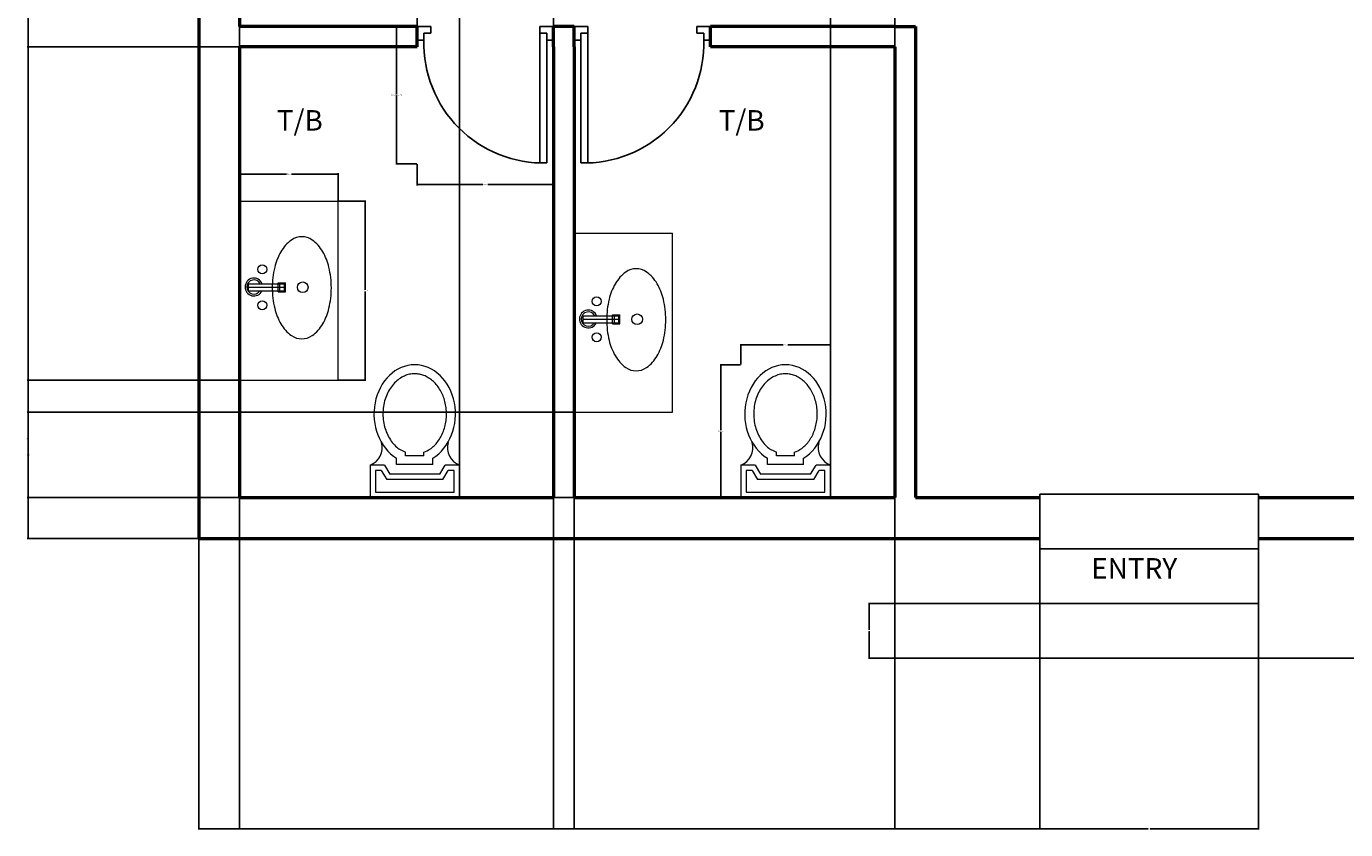
# Model space of a CAD drawing. Units: inches. Extents: x 1865 to 2541, y 1997 to 2759.
# Tile 1 of 11: x 1865 to 2155, y 1997 to 2174. Entities that reach past the tile are written whole.
import ezdxf

# ---------------------------------------------------------------- set-up
doc = ezdxf.new("R2010")
doc.units = ezdxf.units.IN
for name, color, linetype, lineweight in [('A-ANNO-DIMS', 2, 'Continuous', 18), ('A-AREA-IDEN', 4, 'Continuous', 18), ('A-FLOR-FIXT', 9, 'Continuous', 18), ('A-WALL', 7, 'Continuous', 50), ('DOOR', 1, 'Continuous', 25), ('STAIRCASE', 2, 'Continuous', 25), ('TEXT', 4, 'Continuous', 18)]:
    doc.layers.add(name, color=color, linetype=linetype, lineweight=lineweight)
doc.styles.get("Standard").update_dxf_attribs({"font": 'arial.ttf'})
doc.dimstyles.get("Standard").update_dxf_attribs({"dimtxt": 0.18, "dimasz": 0.18, "dimexe": 0.18, "dimexo": 0.0625, "dimgap": 0.09, "dimtad": 0, "dimtih": 1, "dimtoh": 1, "dimdec": 4, "dimzin": 0, "dimdsep": 46, "dimtxsty": 'Standard', "dimcen": 0.09, "dimadec": 0, "dimazin": 0, "dimtfac": 1, "dimtdec": 4, "dimtofl": 0, "dimtmove": 0, "dimatfit": 3, "dimfxl": 1, "dimtolj": 1, "dimtzin": 0, "dimarcsym": 0})

# ---------------------------------------------------------------- blocks, each defined once
blk = doc.blocks.new('A$C50A015BB')
for p, q in [((0, 0.55), (1, 0.55)), ((0, 0.55), (0, 0)), ((1, 0.55), (1, 0)), ((0.4985, 0.5), (0.5385, 0.5)), ((0.4985, 0.5), (0.4985, 0.3)), ((0.5185, 0.5), (0.5185, 0.3)), ((0.5385, 0.5), (0.5385, 0.3)), ((0.4935, 0.335), (0.4935, 0.295)), ((0.4935, 0.335), (0.5435, 0.335)), ((0.4935, 0.295), (0.5435, 0.295)), ((0.4985, 0.325), (0.5385, 0.325)), ((0.4985, 0.3), (0.5385, 0.3)), ((0.5435, 0.335), (0.5435, 0.295)), ((0, 0), (1, 0)), ((0, 0), (1, 0))]:
    blk.add_line(p, q)
for centre, radius in [((0.4185, 0.424), 0.025), ((0.6185, 0.424), 0.025), ((0.5185, 0.1981), 0.0298)]:
    blk.add_circle(centre, radius)
for centre, radius, start, end in [((0.5201, 0.4703), 0.0497, 291.74253, 244.23308), ((0.5201, 0.4703), 0.0397, 297.63203, 237.02558), ((0.4185, 0.1397), 0.2081, 120.06859, 144.41781), ((0.4772, 0.0383), 0.3252, 103.48533, 120.06859), ((0.5157, -0.1225), 0.4906, 90, 103.48533), ((0.5157, -0.1225), 0.4906, 76.51467, 90), ((0.5543, 0.0383), 0.3252, 59.93141, 76.51467), ((0.613, 0.1397), 0.2081, 35.58219, 59.93141), ((0.3299, 0.2031), 0.0991, 144.41781, 180), ((0.7016, 0.2031), 0.0991, 0, 35.58219), ((0.3299, 0.2031), 0.0991, 180, 215.58219), ((0.7016, 0.2031), 0.0991, 324.41781, 0), ((0.4185, 0.2665), 0.2081, 215.58219, 239.93141), ((0.4772, 0.3679), 0.3252, 239.93141, 256.51467), ((0.5543, 0.3679), 0.3252, 283.48533, 300.06859), ((0.613, 0.2665), 0.2081, 300.06859, 324.41781), ((0.5157, 0.5288), 0.4906, 256.51467, 270), ((0.5157, 0.5288), 0.4906, 270, 283.48533)]:
    blk.add_arc(centre, radius, start, end)
blk = doc.blocks.new('A$C7C8779AE')
for p, q in [((0, 0.7405), (0, 0.5605)), ((0.5, 0.7405), (0, 0.7405)), ((0.5, 0.5605), (0.5, 0.7405)), ((0.47, 0.7105), (0.03, 0.7105)), ((0.03, 0.7105), (0.03, 0.5905)), ((0.47, 0.5905), (0.47, 0.7105)), ((0.03, 0.5905), (0.063, 0.5905)), ((0.093, 0.6405), (0.063, 0.5905)), ((0.11, 0.6105), (0.08, 0.5605)), ((0.093, 0.6405), (0.407, 0.6405)), ((0.11, 0.6105), (0.39, 0.6105)), ((0.42, 0.5605), (0.39, 0.6105)), ((0.437, 0.5905), (0.407, 0.6405)), ((0.437, 0.5905), (0.47, 0.5905)), ((0, 0.5605), (0.08, 0.5605)), ((0.1497, 0.557), (0.1497, 0.5203)), ((0.1497, 0.557), (0.3514, 0.557)), ((0.3514, 0.557), (0.3514, 0.5203)), ((0.42, 0.5605), (0.5, 0.5605)), ((0.1997, 0.507), (0.1997, 0.4879)), ((0.1997, 0.507), (0.3014, 0.507)), ((0.3014, 0.507), (0.3014, 0.4879))]:
    blk.add_line(p, q)
for centre, start, end in [((-0.0386, 0.4613), 344.64203, 68.73386), ((0.5386, 0.4613), 111.26614, 195.35797)]:
    blk.add_arc(centre, 0.1064, start, end)
blk.add_ellipse((0.2506, 0.2744), major_axis=(0, 0.2744), ratio=0.828948, start_param=0.459479, end_param=5.823706)
blk.add_open_spline([(0.1997, 0.4879), (0.1697, 0.474), (0.1642, 0.4702), (0.1512, 0.4602), (0.1438, 0.4535), (0.1298, 0.4388), (0.1233, 0.4306), (0.1111, 0.4131), (0.1055, 0.4037), (0.0956, 0.3838), (0.0912, 0.3733), (0.0838, 0.3516), (0.0808, 0.3403), (0.0762, 0.3172), (0.0746, 0.3055), (0.073, 0.2817), (0.0729, 0.2698), (0.0743, 0.246), (0.0758, 0.2342), (0.0801, 0.2111), (0.0831, 0.1998), (0.0903, 0.1779), (0.0945, 0.1673), (0.1043, 0.1473), (0.1098, 0.1378), (0.1218, 0.12), (0.1283, 0.1118), (0.1421, 0.0968), (0.1494, 0.09), (0.1646, 0.078), (0.1725, 0.0728), (0.1887, 0.064), (0.1969, 0.0603), (0.2137, 0.0547), (0.2222, 0.0527), (0.2392, 0.0502), (0.2478, 0.0498), (0.2664, 0.0505), (0.2764, 0.052), (0.2963, 0.0573), (0.3061, 0.061), (0.3253, 0.0707), (0.3346, 0.0766), (0.3525, 0.0906), (0.3611, 0.0987), (0.3771, 0.1169), (0.3845, 0.127), (0.3978, 0.1488), (0.4037, 0.1605), (0.4137, 0.1853), (0.4178, 0.1983), (0.424, 0.2251), (0.4261, 0.2389), (0.4282, 0.2668), (0.4283, 0.2809), (0.4262, 0.3088), (0.4241, 0.3226), (0.418, 0.3495), (0.414, 0.3625), (0.404, 0.3873), (0.3982, 0.3991), (0.385, 0.421), (0.3776, 0.4311), (0.3617, 0.4494), (0.3531, 0.4575), (0.3382, 0.4693), (0.3321, 0.4736), (0.3014, 0.4879)], degree=3, knots=[0.459479, 0.459479, 0.459479, 0.459479, 0.567422, 0.567422, 0.720865, 0.720865, 0.874307, 0.874307, 1.02775, 1.02775, 1.181192, 1.181192, 1.334635, 1.334635, 1.488077, 1.488077, 1.64152, 1.64152, 1.794963, 1.794963, 1.948405, 1.948405, 2.101848, 2.101848, 2.25529, 2.25529, 2.408733, 2.408733, 2.562175, 2.562175, 2.715618, 2.715618, 2.86906, 2.86906, 3.022503, 3.022503, 3.175946, 3.175946, 3.356457, 3.356457, 3.536968, 3.536968, 3.717479, 3.717479, 3.89799, 3.89799, 4.078501, 4.078501, 4.259012, 4.259012, 4.439523, 4.439523, 4.620035, 4.620035, 4.800546, 4.800546, 4.981057, 4.981057, 5.161568, 5.161568, 5.342079, 5.342079, 5.52259, 5.52259, 5.703101, 5.703101, 5.823706, 5.823706, 5.823706, 5.823706])
blk = doc.blocks.new('DOOR-SWING-30IN')
for p, q in [((3, 30), (0, 30)), ((0, 30), (0, 27)), ((3, 28.5), (3, 30)), ((0, 27), (1.5, 27)), ((0, 27), (30, 27)), ((1.5, 27), (1.5, 28.5)), ((1.5, 28.5), (3, 28.5)), ((1.5, 28.5), (30, 28.5)), ((0, 0), (0, 3)), ((0, 3), (1.5, 3)), ((1.5, 3), (1.5, 1.5)), ((1.5, 1.5), (3, 1.5)), ((3, 1.5), (3, 0)), ((3, 0), (0, 0))]:
    blk.add_line(p, q)
blk.add_arc((3.75, 27.75), 26.26, 268.3634, 1.6366)
blk = doc.blocks.new('*D30')
at = {"layer": 'A-ANNO-DIMS', "color": 0, "lineweight": -2, "transparency": 16777216}
for p, q in [((1933.96, 2135.58), (1939.98, 2135.58)), ((1939.8, 2135.4), (1939.8, 2116.08)), ((1939.8, 2096.39), (1939.8, 2115.72)), ((1933.96, 2096.21), (1939.98, 2096.21))]:
    blk.add_line(p, q, dxfattribs=at)
at = {"layer": 'A-ANNO-DIMS', "color": 0, "transparency": 16777216}
for points in [[(1939.77, 2135.4), (1939.83, 2135.4), (1939.8, 2135.58)], [(1939.77, 2096.39), (1939.83, 2096.39), (1939.8, 2096.21)]]:
    blk.add_solid(points, dxfattribs=at)
at = {"layer": 'Defpoints', "color": 0, "transparency": 16777216}
for p in [(1933.9, 2135.58), (1939.8, 2135.58), (1933.9, 2096.21)]:
    blk.add_point(p, dxfattribs=at)
at = {"layer": 'A-ANNO-DIMS', "color": 0, "transparency": 16777216, "insert": (1939.8, 2115.9), "char_height": 0.18, "attachment_point": 5}
blk.add_mtext('\\A1;SINK 39 TYP.', dxfattribs=at)
blk = doc.blocks.new('*D31')
at = {"layer": 'A-ANNO-DIMS', "color": 0, "lineweight": -2, "transparency": 16777216}
for p, q in [((1912.24, 2135.65), (1912.24, 2141.67)), ((1912.42, 2141.49), (1922.54, 2141.49)), ((1933.72, 2141.49), (1923.6, 2141.49)), ((1933.9, 2135.65), (1933.9, 2141.67))]:
    blk.add_line(p, q, dxfattribs=at)
at = {"layer": 'A-ANNO-DIMS', "color": 0, "transparency": 16777216}
for points in [[(1912.42, 2141.52), (1912.42, 2141.46), (1912.24, 2141.49)], [(1933.72, 2141.52), (1933.72, 2141.46), (1933.9, 2141.49)]]:
    blk.add_solid(points, dxfattribs=at)
at = {"layer": 'Defpoints', "color": 0, "transparency": 16777216}
for p in [(1912.24, 2141.49), (1912.24, 2135.58), (1933.9, 2135.58)]:
    blk.add_point(p, dxfattribs=at)
at = {"layer": 'A-ANNO-DIMS', "color": 0, "transparency": 16777216, "insert": (1923.07, 2141.49), "char_height": 0.18, "attachment_point": 5}
blk.add_mtext('\\A1;22 TYP.', dxfattribs=at)
blk = doc.blocks.new('*D32')
at = {"layer": 'A-ANNO-DIMS', "color": 0, "lineweight": -2, "transparency": 16777216}
for p, q in [((1951.18, 2173.95), (1946.53, 2173.95)), ((1946.71, 2173.77), (1946.71, 2159.03)), ((1946.71, 2143.92), (1946.71, 2158.66)), ((1951.18, 2143.74), (1946.53, 2143.74))]:
    blk.add_line(p, q, dxfattribs=at)
at = {"layer": 'A-ANNO-DIMS', "color": 0, "transparency": 16777216}
for points in [[(1946.68, 2173.77), (1946.74, 2173.77), (1946.71, 2173.95)], [(1946.68, 2143.92), (1946.74, 2143.92), (1946.71, 2143.74)]]:
    blk.add_solid(points, dxfattribs=at)
at = {"layer": 'Defpoints', "color": 0, "transparency": 16777216}
for p in [(1951.24, 2173.95), (1946.71, 2143.74), (1951.24, 2143.74)]:
    blk.add_point(p, dxfattribs=at)
at = {"layer": 'A-ANNO-DIMS', "color": 0, "transparency": 16777216, "insert": (1946.71, 2158.85), "char_height": 0.18, "attachment_point": 5}
blk.add_mtext('\\A1;DOOR SWING 30 TYP.', dxfattribs=at)
blk = doc.blocks.new('*D33')
at = {"layer": 'A-ANNO-DIMS', "color": 0, "lineweight": -2, "transparency": 16777216}
for p, q in [((1951.24, 2143.68), (1951.24, 2139.03)), ((1981.24, 2143.68), (1981.24, 2139.03)), ((1951.42, 2139.21), (1965.71, 2139.21)), ((1981.06, 2139.21), (1966.77, 2139.21))]:
    blk.add_line(p, q, dxfattribs=at)
at = {"layer": 'A-ANNO-DIMS', "color": 0, "transparency": 16777216}
for points in [[(1951.42, 2139.24), (1951.42, 2139.18), (1951.24, 2139.21)], [(1981.06, 2139.24), (1981.06, 2139.18), (1981.24, 2139.21)]]:
    blk.add_solid(points, dxfattribs=at)
at = {"layer": 'Defpoints', "color": 0, "transparency": 16777216}
for p in [(1951.24, 2143.74), (1981.24, 2143.74), (1981.24, 2139.21)]:
    blk.add_point(p, dxfattribs=at)
at = {"layer": 'A-ANNO-DIMS', "color": 0, "transparency": 16777216, "insert": (1966.24, 2139.21), "char_height": 0.18, "attachment_point": 5}
blk.add_mtext('\\A1;30 TYP.', dxfattribs=at)
blk = doc.blocks.new('*D34')
at = {"layer": 'A-ANNO-DIMS', "color": 0, "lineweight": -2, "transparency": 16777216}
for p, q in [((2022.32, 2099.6), (2017.83, 2099.6)), ((2018.01, 2099.42), (2018.01, 2085.21)), ((2018.01, 2070.63), (2018.01, 2084.84)), ((2022.32, 2070.45), (2017.83, 2070.45))]:
    blk.add_line(p, q, dxfattribs=at)
at = {"layer": 'A-ANNO-DIMS', "color": 0, "transparency": 16777216}
for points in [[(2017.98, 2099.42), (2018.04, 2099.42), (2018.01, 2099.6)], [(2017.98, 2070.63), (2018.04, 2070.63), (2018.01, 2070.45)]]:
    blk.add_solid(points, dxfattribs=at)
at = {"layer": 'Defpoints', "color": 0, "transparency": 16777216}
for p in [(2022.38, 2099.6), (2018.01, 2070.45), (2022.38, 2070.45)]:
    blk.add_point(p, dxfattribs=at)
at = {"layer": 'A-ANNO-DIMS', "color": 0, "transparency": 16777216, "insert": (2018.01, 2085.03), "char_height": 0.18, "attachment_point": 5}
blk.add_mtext('\\A1;WC 29 TYP.', dxfattribs=at)
blk = doc.blocks.new('*D35')
at = {"layer": 'A-ANNO-DIMS', "color": 0, "lineweight": -2, "transparency": 16777216}
for p, q in [((2022.38, 2099.66), (2022.38, 2104.15)), ((2022.56, 2103.97), (2031.69, 2103.97)), ((2041.89, 2103.97), (2032.75, 2103.97)), ((2042.07, 2099.66), (2042.07, 2104.15))]:
    blk.add_line(p, q, dxfattribs=at)
at = {"layer": 'A-ANNO-DIMS', "color": 0, "transparency": 16777216}
for points in [[(2022.56, 2104), (2022.56, 2103.94), (2022.38, 2103.97)], [(2041.89, 2104), (2041.89, 2103.94), (2042.07, 2103.97)]]:
    blk.add_solid(points, dxfattribs=at)
at = {"layer": 'Defpoints', "color": 0, "transparency": 16777216}
for p in [(2022.38, 2103.97), (2022.38, 2099.6), (2042.07, 2099.6)]:
    blk.add_point(p, dxfattribs=at)
at = {"layer": 'A-ANNO-DIMS', "color": 0, "transparency": 16777216, "insert": (2032.22, 2103.97), "char_height": 0.18, "attachment_point": 5}
blk.add_mtext('\\A1;20 TYP.', dxfattribs=at)
blk = doc.blocks.new('*D41')
at = {"layer": 'A-ANNO-DIMS', "color": 0, "lineweight": -2, "transparency": 16777216}
for p, q in [((2503.31, 2721.45), (2540.92, 2721.45)), ((2540.74, 2721.27), (2540.74, 2378.49)), ((2540.74, 2035.35), (2540.74, 2378.13)), ((2136.19, 2035.17), (2540.92, 2035.17))]:
    blk.add_line(p, q, dxfattribs=at)
at = {"layer": 'A-ANNO-DIMS', "color": 0, "transparency": 16777216}
for points in [[(2540.71, 2721.27), (2540.77, 2721.27), (2540.74, 2721.45)], [(2540.71, 2035.35), (2540.77, 2035.35), (2540.74, 2035.17)]]:
    blk.add_solid(points, dxfattribs=at)
at = {"layer": 'Defpoints', "color": 0, "transparency": 16777216}
for p in [(2503.24, 2721.45), (2136.13, 2035.17), (2540.74, 2035.17)]:
    blk.add_point(p, dxfattribs=at)
at = {"layer": 'A-ANNO-DIMS', "color": 0, "transparency": 16777216, "insert": (2540.74, 2378.31), "char_height": 0.18, "attachment_point": 5}
blk.add_mtext('\\A1;686.3', dxfattribs=at)
blk = doc.blocks.new('*D42')
at = {"layer": 'A-ANNO-DIMS', "color": 0, "lineweight": -2, "transparency": 16777216}
for p, q in [((1903.18, 2721.45), (1865.56, 2721.45)), ((1865.74, 2721.27), (1865.74, 2391.63)), ((1865.74, 2061.63), (1865.74, 2391.27)), ((1903.18, 2061.45), (1865.56, 2061.45))]:
    blk.add_line(p, q, dxfattribs=at)
at = {"layer": 'A-ANNO-DIMS', "color": 0, "transparency": 16777216}
for points in [[(1865.71, 2721.27), (1865.77, 2721.27), (1865.74, 2721.45)], [(1865.71, 2061.63), (1865.77, 2061.63), (1865.74, 2061.45)]]:
    blk.add_solid(points, dxfattribs=at)
at = {"layer": 'Defpoints', "color": 0, "transparency": 16777216}
for p in [(1865.74, 2721.45), (1903.24, 2721.45), (1903.24, 2061.45)]:
    blk.add_point(p, dxfattribs=at)
at = {"layer": 'A-ANNO-DIMS', "color": 0, "transparency": 16777216, "insert": (1865.74, 2391.45), "char_height": 0.18, "attachment_point": 5}
blk.add_mtext('\\A1;660', dxfattribs=at)
blk = doc.blocks.new('*D51')
at = {"layer": 'A-ANNO-DIMS', "color": 0, "lineweight": -2, "transparency": 16777216}
for p, q in [((1912.18, 2169.45), (1865.56, 2169.45)), ((1865.74, 2169.27), (1865.74, 2120.13)), ((1865.74, 2070.63), (1865.74, 2119.77)), ((1912.18, 2070.45), (1865.56, 2070.45))]:
    blk.add_line(p, q, dxfattribs=at)
at = {"layer": 'A-ANNO-DIMS', "color": 0, "transparency": 16777216}
for points in [[(1865.71, 2169.27), (1865.77, 2169.27), (1865.74, 2169.45)], [(1865.71, 2070.63), (1865.77, 2070.63), (1865.74, 2070.45)]]:
    blk.add_solid(points, dxfattribs=at)
at = {"layer": 'Defpoints', "color": 0, "transparency": 16777216}
for p in [(1912.24, 2169.45), (1865.74, 2070.45), (1912.24, 2070.45)]:
    blk.add_point(p, dxfattribs=at)
at = {"layer": 'A-ANNO-DIMS', "color": 0, "transparency": 16777216, "insert": (1865.74, 2119.95), "char_height": 0.18, "attachment_point": 5}
blk.add_mtext('\\A1;99', dxfattribs=at)
blk = doc.blocks.new('*D52')
at = {"layer": 'A-ANNO-DIMS', "color": 0, "lineweight": -2, "transparency": 16777216}
for p, q in [((1912.24, 2070.39), (1912.24, 1997.49)), ((1981.24, 2070.39), (1981.24, 1997.49)), ((1912.42, 1997.67), (1946.52, 1997.67)), ((1981.06, 1997.67), (1946.96, 1997.67))]:
    blk.add_line(p, q, dxfattribs=at)
at = {"layer": 'A-ANNO-DIMS', "color": 0, "transparency": 16777216}
for points in [[(1912.42, 1997.7), (1912.42, 1997.64), (1912.24, 1997.67)], [(1981.06, 1997.7), (1981.06, 1997.64), (1981.24, 1997.67)]]:
    blk.add_solid(points, dxfattribs=at)
at = {"layer": 'Defpoints', "color": 0, "transparency": 16777216}
for p in [(1912.24, 2070.45), (1981.24, 2070.45), (1981.24, 1997.67)]:
    blk.add_point(p, dxfattribs=at)
at = {"layer": 'A-ANNO-DIMS', "color": 0, "transparency": 16777216, "insert": (1946.74, 1997.67), "char_height": 0.18, "attachment_point": 5}
blk.add_mtext('\\A1;69', dxfattribs=at)
blk = doc.blocks.new('*D53')
at = {"layer": 'A-ANNO-DIMS', "color": 0, "lineweight": -2, "transparency": 16777216}
for p, q in [((1985.74, 2070.39), (1985.74, 1997.49)), ((2056.24, 2070.39), (2056.24, 1997.49)), ((1985.92, 1997.67), (2020.67, 1997.67)), ((2056.06, 1997.67), (2021.32, 1997.67))]:
    blk.add_line(p, q, dxfattribs=at)
at = {"layer": 'A-ANNO-DIMS', "color": 0, "transparency": 16777216}
for points in [[(1985.92, 1997.7), (1985.92, 1997.64), (1985.74, 1997.67)], [(2056.06, 1997.7), (2056.06, 1997.64), (2056.24, 1997.67)]]:
    blk.add_solid(points, dxfattribs=at)
at = {"layer": 'Defpoints', "color": 0, "transparency": 16777216}
for p in [(1985.74, 2070.45), (2056.24, 2070.45), (2056.24, 1997.67)]:
    blk.add_point(p, dxfattribs=at)
at = {"layer": 'A-ANNO-DIMS', "color": 0, "transparency": 16777216, "insert": (2020.99, 1997.67), "char_height": 0.18, "attachment_point": 5}
blk.add_mtext('\\A1;70.5', dxfattribs=at)
blk = doc.blocks.new('*D57')
at = {"layer": 'A-ANNO-DIMS', "color": 0, "lineweight": -2, "transparency": 16777216}
for p, q in [((1903.24, 2061.39), (1903.24, 1997.49)), ((2088.13, 2061.39), (2088.13, 1997.49)), ((1903.42, 1997.67), (1995.3, 1997.67)), ((2087.95, 1997.67), (1996.07, 1997.67))]:
    blk.add_line(p, q, dxfattribs=at)
at = {"layer": 'A-ANNO-DIMS', "color": 0, "transparency": 16777216}
for points in [[(1903.42, 1997.7), (1903.42, 1997.64), (1903.24, 1997.67)], [(2087.95, 1997.7), (2087.95, 1997.64), (2088.13, 1997.67)]]:
    blk.add_solid(points, dxfattribs=at)
at = {"layer": 'Defpoints', "color": 0, "transparency": 16777216}
for p in [(1903.24, 2061.45), (2088.13, 2061.45), (2088.13, 1997.67)]:
    blk.add_point(p, dxfattribs=at)
at = {"layer": 'A-ANNO-DIMS', "color": 0, "transparency": 16777216, "insert": (1995.69, 1997.67), "char_height": 0.18, "attachment_point": 5}
blk.add_mtext('\\A1;184.9', dxfattribs=at)
blk = doc.blocks.new('*D58')
at = {"layer": 'A-ANNO-DIMS', "color": 0, "lineweight": -2, "transparency": 16777216}
for p, q in [((2088.13, 2035.11), (2088.13, 1997.49)), ((2136.13, 2035.11), (2136.13, 1997.49)), ((2088.31, 1997.67), (2111.91, 1997.67)), ((2135.95, 1997.67), (2112.35, 1997.67))]:
    blk.add_line(p, q, dxfattribs=at)
at = {"layer": 'A-ANNO-DIMS', "color": 0, "transparency": 16777216}
for points in [[(2088.31, 1997.7), (2088.31, 1997.64), (2088.13, 1997.67)], [(2135.95, 1997.7), (2135.95, 1997.64), (2136.13, 1997.67)]]:
    blk.add_solid(points, dxfattribs=at)
at = {"layer": 'Defpoints', "color": 0, "transparency": 16777216}
for p in [(2088.13, 2035.17), (2136.13, 2035.17), (2136.13, 1997.67)]:
    blk.add_point(p, dxfattribs=at)
at = {"layer": 'A-ANNO-DIMS', "color": 0, "transparency": 16777216, "insert": (2112.13, 1997.67), "char_height": 0.18, "attachment_point": 5}
blk.add_mtext('\\A1;48', dxfattribs=at)
blk = doc.blocks.new('*D68')
at = {"layer": 'A-ANNO-DIMS', "color": 0, "lineweight": -2, "transparency": 16777216}
for p, q in [((1912.24, 2169.51), (1912.24, 2759.13)), ((1912.42, 2758.95), (1931.52, 2758.95)), ((1951.06, 2758.95), (1931.96, 2758.95)), ((1951.24, 2169.51), (1951.24, 2759.13))]:
    blk.add_line(p, q, dxfattribs=at)
at = {"layer": 'A-ANNO-DIMS', "color": 0, "transparency": 16777216}
for points in [[(1912.42, 2758.98), (1912.42, 2758.92), (1912.24, 2758.95)], [(1951.06, 2758.98), (1951.06, 2758.92), (1951.24, 2758.95)]]:
    blk.add_solid(points, dxfattribs=at)
at = {"layer": 'Defpoints', "color": 0, "transparency": 16777216}
for p in [(1951.24, 2758.95), (1912.24, 2169.45), (1951.24, 2169.45)]:
    blk.add_point(p, dxfattribs=at)
at = {"layer": 'A-ANNO-DIMS', "color": 0, "transparency": 16777216, "insert": (1931.74, 2758.95), "char_height": 0.18, "attachment_point": 5}
blk.add_mtext('\\A1;39', dxfattribs=at)
blk = doc.blocks.new('*D75')
at = {"layer": 'A-ANNO-DIMS', "color": 0, "lineweight": -2, "transparency": 16777216}
for p, q in [((1912.18, 2096.21), (1865.56, 2096.21)), ((1865.74, 2096.03), (1865.74, 2083.51)), ((1865.74, 2070.63), (1865.74, 2083.15)), ((1912.18, 2070.45), (1865.56, 2070.45))]:
    blk.add_line(p, q, dxfattribs=at)
at = {"layer": 'A-ANNO-DIMS', "color": 0, "transparency": 16777216}
for points in [[(1865.71, 2096.03), (1865.77, 2096.03), (1865.74, 2096.21)], [(1865.71, 2070.63), (1865.77, 2070.63), (1865.74, 2070.45)]]:
    blk.add_solid(points, dxfattribs=at)
at = {"layer": 'Defpoints', "color": 0, "transparency": 16777216}
for p in [(1912.24, 2096.21), (1865.74, 2070.45), (1912.24, 2070.45)]:
    blk.add_point(p, dxfattribs=at)
at = {"layer": 'A-ANNO-DIMS', "color": 0, "transparency": 16777216, "insert": (1865.74, 2083.33), "char_height": 0.18, "attachment_point": 5}
blk.add_mtext('\\A1;25.764', dxfattribs=at)
blk = doc.blocks.new('*D76')
at = {"layer": 'A-ANNO-DIMS', "color": 0, "lineweight": -2, "transparency": 16777216}
for p, q in [((1985.68, 2089.19), (1865.56, 2089.19)), ((1865.74, 2089.01), (1865.74, 2080)), ((1865.74, 2070.63), (1865.74, 2079.64)), ((1985.68, 2070.45), (1865.56, 2070.45))]:
    blk.add_line(p, q, dxfattribs=at)
at = {"layer": 'A-ANNO-DIMS', "color": 0, "transparency": 16777216}
for points in [[(1865.71, 2089.01), (1865.77, 2089.01), (1865.74, 2089.19)], [(1865.71, 2070.63), (1865.77, 2070.63), (1865.74, 2070.45)]]:
    blk.add_solid(points, dxfattribs=at)
at = {"layer": 'Defpoints', "color": 0, "transparency": 16777216}
for p in [(1985.74, 2089.19), (1865.74, 2070.45), (1985.74, 2070.45)]:
    blk.add_point(p, dxfattribs=at)
at = {"layer": 'A-ANNO-DIMS', "color": 0, "transparency": 16777216, "insert": (1865.74, 2079.82), "char_height": 0.18, "attachment_point": 5}
blk.add_mtext('\\A1;18.737', dxfattribs=at)
blk = doc.blocks.new('*D81')
at = {"layer": 'A-ANNO-DIMS', "color": 0, "lineweight": -2, "transparency": 16777216}
for p, q in [((1960.58, 2070.51), (1960.58, 2759.13)), ((1960.76, 2758.95), (1970.44, 2758.95)), ((1981.06, 2758.95), (1971.38, 2758.95)), ((1981.24, 2070.51), (1981.24, 2759.13))]:
    blk.add_line(p, q, dxfattribs=at)
at = {"layer": 'A-ANNO-DIMS', "color": 0, "transparency": 16777216}
for points in [[(1960.76, 2758.98), (1960.76, 2758.92), (1960.58, 2758.95)], [(1981.06, 2758.98), (1981.06, 2758.92), (1981.24, 2758.95)]]:
    blk.add_solid(points, dxfattribs=at)
at = {"layer": 'Defpoints', "color": 0, "transparency": 16777216}
for p in [(1960.58, 2758.95), (1960.58, 2070.45), (1981.24, 2070.45)]:
    blk.add_point(p, dxfattribs=at)
at = {"layer": 'A-ANNO-DIMS', "color": 0, "transparency": 16777216, "insert": (1970.91, 2758.95), "char_height": 0.18, "attachment_point": 5}
blk.add_mtext('\\A1;20.665', dxfattribs=at)
blk = doc.blocks.new('*D82')
at = {"layer": 'A-ANNO-DIMS', "color": 0, "lineweight": -2, "transparency": 16777216}
for p, q in [((2042.07, 2070.51), (2042.07, 2759.13)), ((2042.25, 2758.95), (2048.7, 2758.95)), ((2056.06, 2758.95), (2049.61, 2758.95)), ((2056.24, 2070.51), (2056.24, 2759.13))]:
    blk.add_line(p, q, dxfattribs=at)
at = {"layer": 'A-ANNO-DIMS', "color": 0, "transparency": 16777216}
for points in [[(2042.25, 2758.98), (2042.25, 2758.92), (2042.07, 2758.95)], [(2056.06, 2758.98), (2056.06, 2758.92), (2056.24, 2758.95)]]:
    blk.add_solid(points, dxfattribs=at)
at = {"layer": 'Defpoints', "color": 0, "transparency": 16777216}
for p in [(2042.07, 2758.95), (2042.07, 2070.45), (2056.24, 2070.45)]:
    blk.add_point(p, dxfattribs=at)
at = {"layer": 'A-ANNO-DIMS', "color": 0, "transparency": 16777216, "insert": (2049.16, 2758.95), "char_height": 0.18, "attachment_point": 5}
blk.add_mtext('\\A1;14.176', dxfattribs=at)
blk = doc.blocks.new('*D83')
at = {"layer": 'A-ANNO-DIMS', "color": 0, "lineweight": -2, "transparency": 16777216}
for p, q in [((2088.07, 2047.17), (2050.45, 2047.17)), ((2050.63, 2046.99), (2050.63, 2041.35)), ((2050.63, 2035.35), (2050.63, 2040.99)), ((2088.07, 2035.17), (2050.45, 2035.17))]:
    blk.add_line(p, q, dxfattribs=at)
at = {"layer": 'A-ANNO-DIMS', "color": 0, "transparency": 16777216}
for points in [[(2050.6, 2046.99), (2050.66, 2046.99), (2050.63, 2047.17)], [(2050.6, 2035.35), (2050.66, 2035.35), (2050.63, 2035.17)]]:
    blk.add_solid(points, dxfattribs=at)
at = {"layer": 'Defpoints', "color": 0, "transparency": 16777216}
for p in [(2050.63, 2047.17), (2088.13, 2047.17), (2088.13, 2035.17)]:
    blk.add_point(p, dxfattribs=at)
at = {"layer": 'A-ANNO-DIMS', "color": 0, "transparency": 16777216, "insert": (2050.63, 2041.17), "char_height": 0.18, "attachment_point": 5}
blk.add_mtext('\\A1;12', dxfattribs=at)

msp = doc.modelspace()

# ---------------------------------------------------------------- linework, layer by layer
at = {"layer": 'A-WALL'}
for p, q in [((1903.243, 2721.4494), (1903.243, 2061.4494)), ((1912.243, 2228.9494), (1912.243, 2173.9494)), ((1951.243, 2173.9494), (1912.243, 2173.9494)), ((1951.243, 2169.4494), (1951.243, 2173.9494)), ((1981.243, 2169.4494), (1981.243, 2173.9494)), ((1985.743, 2173.9494), (1981.243, 2173.9494)), ((1985.743, 2169.4494), (1985.743, 2173.9494)), ((2056.243, 2173.9494), (2015.743, 2173.9494)), ((2015.743, 2169.4494), (2015.743, 2173.9494)), ((2056.243, 2173.9494), (2056.243, 2173.9494)), ((2056.243, 2173.9494), (2060.743, 2173.9494)), ((2060.743, 2173.9494), (2060.743, 2070.4494)), ((1951.243, 2169.4494), (1912.243, 2169.4494)), ((1912.243, 2169.4494), (1912.243, 2070.4494)), ((1981.243, 2169.4494), (1981.243, 2070.4494)), ((1985.743, 2169.4494), (1985.743, 2070.4494)), ((2056.243, 2169.4494), (2015.743, 2169.4494)), ((2056.243, 2169.4494), (2056.243, 2070.4494)), ((1912.243, 2070.4494), (1981.243, 2070.4494)), ((1985.743, 2070.4494), (2056.243, 2070.4494)), ((2060.743, 2070.4494), (2088.1299, 2070.4494)), ((2136.1299, 2070.4494), (2185.243, 2070.4494)), ((1903.243, 2061.4494), (2088.1299, 2061.4494)), ((2136.1299, 2061.4494), (2503.243, 2061.4494))]:
    msp.add_line(p, q, dxfattribs=at)
at = {"layer": 'STAIRCASE'}
for p, q in [((2136.1299, 2071.1708), (2088.1299, 2071.1708)), ((2088.1299, 2071.1708), (2088.1299, 2035.1708)), ((2136.1299, 2035.1708), (2136.1299, 2071.1708)), ((2088.1299, 2059.1708), (2136.1299, 2059.1708)), ((2088.1299, 2047.1708), (2136.1299, 2047.1708)), ((2088.1299, 2035.1708), (2136.1299, 2035.1708))]:
    msp.add_line(p, q, dxfattribs=at)

# ---------------------------------------------------------------- block references
at = {"layer": 'A-FLOR-FIXT', "xscale": 39.37007874015748, "yscale": 39.37007874015748, "zscale": 39.37007874015748}
for name, p, rotation in [('A$C50A015BB', (1933.8965, 2096.2139), 90), ('A$C50A015BB', (2007.3965, 2089.1864), 90), ('A$C7C8779AE', (1960.5785, 2099.6015), 180), ('A$C7C8779AE', (2042.0671, 2099.6015), 180)]:
    msp.add_blockref(name, p, dxfattribs=dict(at, rotation=rotation))
at = {"layer": 'DOOR', "rotation": 269.9999999999956}
msp.add_blockref('DOOR-SWING-30IN', (1951.2434, 2173.9494), dxfattribs=at)
at = {"layer": 'DOOR', "extrusion": (0, 0, -1), "zscale": -1, "rotation": 269.9999999999965}
msp.add_blockref('DOOR-SWING-30IN', (-2015.7426, 2173.9494), dxfattribs=at)

# ---------------------------------------------------------------- texts
at = {"layer": 'A-AREA-IDEN', "char_height": 4.5, "attachment_point": 1}
for insert in [(1920.4004, 2155.5491), (2017.5141, 2155.5491)]:
    msp.add_mtext_dynamic_manual_height_columns('T/B', width=66.075761, gutter_width=12.5, heights=[0], dxfattribs=dict(at, insert=insert))
at = {"layer": 'TEXT', "insert": (2099.3979, 2057.1399), "char_height": 4.5, "attachment_point": 1}
msp.add_mtext_dynamic_manual_height_columns('ENTRY', width=66.075761, gutter_width=12.5, heights=[0], dxfattribs=at)

# ---------------------------------------------------------------- dimensions: what is measured, and where the dimension line sits
at = {"layer": 'A-ANNO-DIMS'}
for base, p1, p2, override, picture, middle in [((1951.243, 2758.9494), (1912.243, 2169.4494), (1951.243, 2169.4494), {"dimdec": 0, "dimlfac": 1, "dimrnd": 0, "dimzin": 0, "dimdsep": 46, "dimlunit": 2}, '*D68', (1931.743, 2758.9494)), ((1960.57848, 2758.94943), (1981.243, 2070.44943), (1960.57848, 2070.44943), {"dimdec": 3, "dimlfac": 1, "dimrnd": 0, "dimzin": 0, "dimdsep": 46, "dimlunit": 2}, '*D81', (1970.91074, 2758.94943)), ((2042.0671, 2758.9494), (2056.243, 2070.4494), (2042.0671, 2070.4494), {"dimdec": 3, "dimlfac": 1, "dimrnd": 0, "dimzin": 0, "dimdsep": 46, "dimlunit": 2}, '*D82', (2049.1551, 2758.9494)), ((1981.243, 1997.6708), (1912.243, 2070.4494), (1981.243, 2070.4494), {"dimdec": 0, "dimlfac": 1, "dimrnd": 0, "dimzin": 0, "dimdsep": 46, "dimlunit": 2}, '*D52', (1946.743, 1997.6708)), ((2056.243, 1997.6708), (1985.743, 2070.4494), (2056.243, 2070.4494), {"dimdec": 1, "dimlfac": 1, "dimrnd": 0, "dimzin": 0, "dimdsep": 46, "dimlunit": 2}, '*D53', (2020.993, 1997.6708)), ((2088.1299, 1997.6708), (1903.243, 2061.4494), (2088.1299, 2061.4494), {"dimdec": 1, "dimlfac": 1, "dimrnd": 0, "dimzin": 0, "dimdsep": 46, "dimlunit": 2}, '*D57', (1995.6865, 1997.6708)), ((2136.1299, 1997.6708), (2088.1299, 2035.1708), (2136.1299, 2035.1708), {"dimdec": 0, "dimlfac": 1, "dimrnd": 0, "dimzin": 0, "dimdsep": 46, "dimlunit": 2}, '*D58', (2112.13, 1997.6708))]:
    dim = msp.add_linear_dim(base=base, p1=p1, p2=p2, dimstyle='Standard', override=override, dxfattribs=at)
    dim.commit()
    dim.dimension.update_dxf_attribs({"geometry": picture, "text_midpoint": middle})
for base, p1, p2, override, picture, middle in [((1865.743, 2721.4494), (1903.243, 2061.4494), (1903.243, 2721.4494), {"dimdec": 0, "dimlfac": 1, "dimrnd": 0, "dimzin": 0, "dimdsep": 46, "dimlunit": 2}, '*D42', (1865.743, 2391.4494)), ((2540.743, 2035.1708), (2503.243, 2721.4494), (2136.1299, 2035.1708), {"dimdec": 1, "dimlfac": 1, "dimrnd": 0, "dimzin": 0, "dimdsep": 46, "dimlunit": 2}, '*D41', (2540.743, 2378.3101)), ((1865.743, 2070.4494), (1912.243, 2169.4494), (1912.243, 2070.4494), {"dimdec": 0, "dimlfac": 1, "dimrnd": 0, "dimzin": 0, "dimdsep": 46, "dimlunit": 2}, '*D51', (1865.743, 2119.9494)), ((1865.742996, 2070.449427), (1912.242996, 2096.213925), (1912.242996, 2070.449427), {"dimdec": 3, "dimlfac": 1, "dimrnd": 0, "dimzin": 0, "dimdsep": 46, "dimlunit": 2}, '*D75', (1865.742996, 2083.331676)), ((1865.743, 2070.4494), (1985.743, 2089.1864), (1985.743, 2070.4494), {"dimdec": 3, "dimlfac": 1, "dimrnd": 0, "dimzin": 0, "dimdsep": 46, "dimlunit": 2}, '*D76', (1865.743, 2079.8179)), ((2050.63, 2047.1708), (2088.1299, 2035.1708), (2088.1299, 2047.1708), {"dimdec": 0, "dimlfac": 1, "dimrnd": 0, "dimzin": 0, "dimdsep": 46, "dimlunit": 2}, '*D83', (2050.63, 2041.1708))]:
    dim = msp.add_linear_dim(base=base, p1=p1, p2=p2, angle=90, dimstyle='Standard', override=override, dxfattribs=at)
    dim.commit()
    dim.dimension.update_dxf_attribs({"geometry": picture, "text_midpoint": middle})
for base, p1, p2, angle, text, picture, middle in [((1946.712, 2143.7431), (1951.243, 2173.9494), (1951.243, 2143.7431), 270, 'DOOR SWING <> TYP.', '*D32', (1946.712, 2158.8463)), ((1912.243, 2141.4895), (1933.8965, 2135.584), (1912.243, 2135.584), 180, '<> TYP.', '*D31', (1923.0698, 2141.4895)), ((1939.8021, 2135.584), (1933.8965, 2096.2139), (1933.8965, 2135.584), 90, 'SINK <> TYP.', '*D30', (1939.8021, 2115.899)), ((2022.3821, 2103.9743), (2042.0671, 2099.6015), (2022.3821, 2099.6015), 180, '<> TYP.', '*D35', (2032.2246, 2103.9743)), ((2018.0093, 2070.4494), (2022.3821, 2099.6015), (2022.3821, 2070.4494), 270, 'WC <> TYP.', '*D34', (2018.0093, 2085.0255))]:
    dim = msp.add_linear_dim(base=base, p1=p1, p2=p2, angle=angle, text=text, dimstyle='Standard', override={"dimdec": 0, "dimlfac": 1, "dimrnd": 0, "dimzin": 0, "dimdsep": 46, "dimlunit": 2}, dxfattribs=at)
    dim.commit()
    dim.dimension.update_dxf_attribs({"geometry": picture, "text_midpoint": middle})
dim = msp.add_linear_dim(base=(1981.243, 2139.2121), p1=(1951.243, 2143.7431), p2=(1981.243, 2143.7431), text='<> TYP.', dimstyle='Standard', override={"dimdec": 0, "dimlfac": 1, "dimrnd": 0, "dimzin": 0, "dimdsep": 46, "dimlunit": 2}, dxfattribs=at)
dim.commit()
dim.dimension.update_dxf_attribs({"geometry": '*D33', "text_midpoint": (1966.243, 2139.2121)})

doc.saveas('drawing.dxf')
